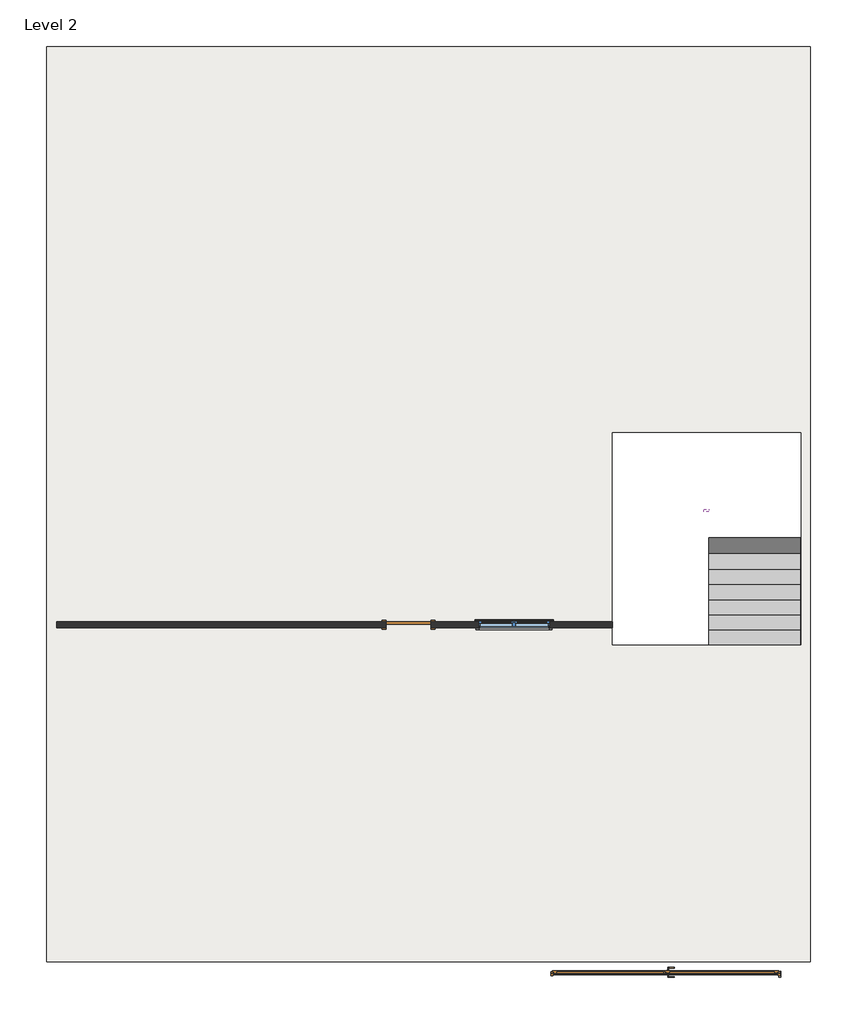
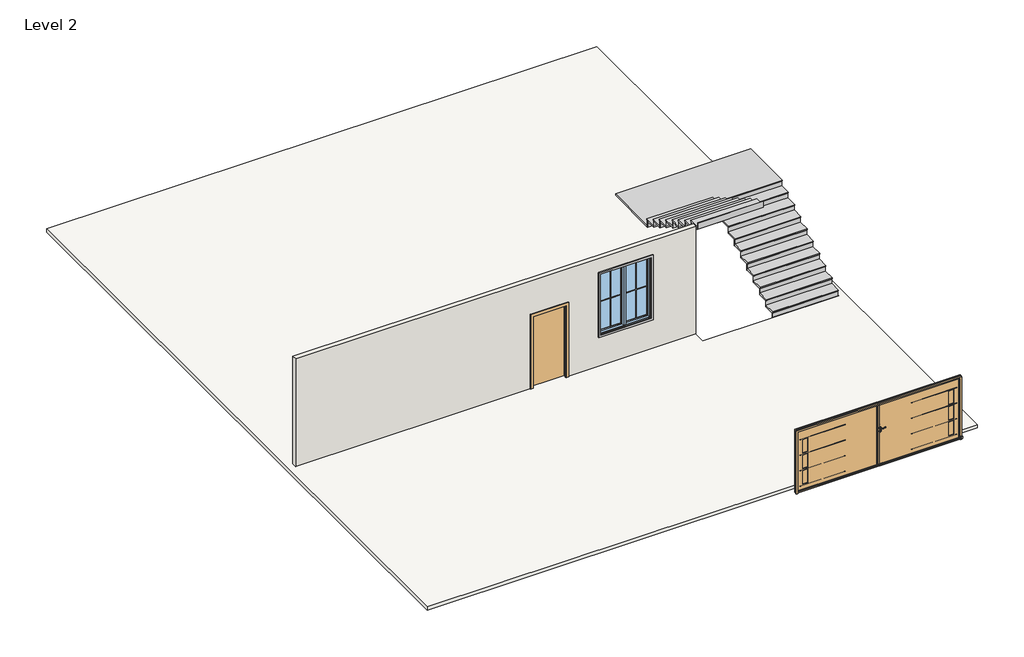
# One storey, incomplete: 4 proxies, 2 doors, 2 walls, 1 member, 1 slab, 1 stair flight, 1 window.
"""IFC4 building model written with IfcOpenShell, lengths in millimetres."""

from ifc_helpers import new_model, si_unit, frame, origin, place, context, project, spatial, polyline, outline, extrude, transform, mapped, element, save
from components import muntin_pattern_2x2_muntin_pattern_2x2_bff912c5, muntin_pattern_2x2_muntin_pattern_2x2_c2194282, trim_window_exterior_flat_with_sill_a4fd29d2, trim_window_interior_flat_picture_frame_640e2092, door_2a186d26, door_a3eb833a, stair_flight_26a2e14d, window_01a3843f

model = new_model("IFC4")

# Units and contexts
model_context = context("Model", 3, world=origin())
ifc_project = project(units=[si_unit("LENGTHUNIT", "METRE", prefix="MILLI")], contexts=[model_context])

# Site, building, storey
site = spatial("IfcSite", under=ifc_project)
building = spatial("IfcBuilding", under=site)
storey = spatial("IfcBuildingStorey", under=building, Name="Level 2", Elevation=762.0)

# Proxies
placement = place(None, origin())
muntin_pattern_2x2_muntin_pattern_2x2_shape = muntin_pattern_2x2_muntin_pattern_2x2_bff912c5(model_context)
element("IfcBuildingElementProxy", 1, Name="Muntin Pattern_2x2 : Muntin Pattern_2x2", ObjectType="Muntin Pattern_2x2 : Muntin Pattern_2x2", at=placement, inside=storey, context=model_context, shape_type="MappedRepresentation", body=[
    mapped(muntin_pattern_2x2_muntin_pattern_2x2_shape, transform((1639.5268946, -8189.1580955, 1746.25), x_axis=(1.0, 0.0, 0.0), y_axis=(0.0, 1.0, 0.0), z_axis=(0.0, 0.0, 1.0))),
])
muntin_pattern_2x2_muntin_pattern_2x2_2_shape = muntin_pattern_2x2_muntin_pattern_2x2_c2194282(model_context)
element("IfcBuildingElementProxy", 2, Name="Muntin Pattern_2x2 : Muntin Pattern_2x2", ObjectType="Muntin Pattern_2x2 : Muntin Pattern_2x2", at=placement, inside=storey, context=model_context, shape_type="MappedRepresentation", body=[
    mapped(muntin_pattern_2x2_muntin_pattern_2x2_2_shape, transform((2360.2518946, -8189.1580955, 1746.25), x_axis=(-1.0, 0.0, 0.0), y_axis=(0.0, -1.0, 0.0), z_axis=(0.0, 0.0, 1.0))),
])
trim_window_exterior_flat_with_sill_shape = trim_window_exterior_flat_with_sill_a4fd29d2(model_context)
element("IfcBuildingElementProxy", 3, Name="Trim-Window-Exterior-Flat : with Sill", ObjectType="Trim-Window-Exterior-Flat : with Sill", at=placement, inside=storey, context=model_context, shape_type="MappedRepresentation", body=[
    mapped(trim_window_exterior_flat_with_sill_shape, transform((1999.8893946, -8179.6330955, 3505.2), x_axis=(1.0, 0.0, 0.0), y_axis=(0.0, 0.0, -1.0), z_axis=(0.0, 1.0, 0.0))),
])
trim_window_interior_flat_picture_frame_shape = trim_window_interior_flat_picture_frame_640e2092(model_context)
element("IfcBuildingElementProxy", 4, Name="Trim-Window-Interior-Flat : Picture Frame", ObjectType="Trim-Window-Interior-Flat : Picture Frame", at=placement, inside=storey, context=model_context, shape_type="MappedRepresentation", body=[
    mapped(trim_window_interior_flat_picture_frame_shape, transform((1999.8893946, -8306.6330955, 3505.2), x_axis=(-1.0, 0.0, 0.0), y_axis=(0.0, 0.0, -1.0), z_axis=(0.0, -1.0, 0.0))),
])

# Doors
door_shape = door_2a186d26(model_context)
element("IfcDoor", 5, at=placement, inside=storey, context=model_context, shape_type="MappedRepresentation", body=[
    mapped(door_shape, transform((5061.1313124, -15304.3330955, 711.2), x_axis=(1.0, 0.0, 0.0), y_axis=(0.0, 1.0, 0.0), z_axis=(0.0, 0.0, 1.0))),
])
door_2_shape = door_a3eb833a(model_context)
element("IfcDoor", 6, ObjectType="Single-Flush : 36\" x 84\"", at=placement, inside=storey, context=model_context, shape_type="MappedRepresentation", body=[
    mapped(door_2_shape, transform((-133.7106054, -8243.1330955, 762.0), x_axis=(-1.0, 0.0, 0.0), y_axis=(0.0, -1.0, 0.0), z_axis=(0.0, 0.0, 1.0))),
])

# Member
element("IfcMember", 7, ObjectType="Stringer - 2\" Width", at=placement, inside=storey, context=model_context, shape_type="SweptSolid", body=[
    extrude(outline(polyline([(5940.6255016, -5904.9976656), (5940.6255016, -5955.7976656), (5839.0255016, -5955.7976656), (5839.0255016, -5904.9976656), (5940.6255016, -5904.9976656)])), frame((0.0, 0.0, 2311.4), z_axis=(0.0, 0.0, 1.0), x_axis=(1.0, 0.0, 0.0)), (0.0, 0.0, 1.0), 304.8),
])

# Slab
element("IfcSlab", 8, ObjectType="Generic - 4\"", at=placement, inside=storey, context=model_context, shape_type="SweptSolid", body=[
    extrude(outline(polyline([(-7454.7186876, -15050.3330955), (-7454.7186876, 3440.8669045), (7988.4813124, 3440.8669045), (7988.4813124, -15050.3330955), (-7454.7186876, -15050.3330955)]), holes=[polyline([(7797.9813124, -4367.7173694), (3981.0893946, -4367.7173694), (3981.0893946, -8648.1976656), (7797.9813124, -8648.1976656), (7797.9813124, -4367.7173694)])]), frame((0.0, 0.0, 660.4), z_axis=(0.0, 0.0, 1.0), x_axis=(1.0, 0.0, 0.0)), (0.0, 0.0, 1.0), 101.6),
])

# Stair flight
stair_flight_shape = stair_flight_26a2e14d(model_context)
element("IfcStairFlight", 9, ObjectType="2\" Tread 1\" Nosing 1/4\" Riser", at=placement, inside=storey, context=model_context, shape_type="MappedRepresentation", body=[
    mapped(stair_flight_shape, transform((0.0, 0.0, 0.0), x_axis=(1.0, 0.0, 0.0), y_axis=(0.0, 1.0, 0.0), z_axis=(0.0, 0.0, 1.0))),
])

# Walls
element("IfcWall", 10, ObjectType="Generic - 5\"", at=placement, inside=storey, context=model_context, shape_type="SweptSolid", body=[
    extrude(outline(polyline([(762.0, -7251.5186876), (762.0, -590.9106054), (2895.6, -590.9106054), (2895.6, 323.4893946), (762.0, 323.4893946), (762.0, 3981.0893946), (3962.4, 3981.0893946), (3962.4, -7251.5186876), (762.0, -7251.5186876)]), holes=[polyline([(3505.2, 1275.9893946), (3505.2, 2723.7893946), (1676.4, 2723.7893946), (1676.4, 1275.9893946), (3505.2, 1275.9893946)])]), frame((0.0, -8306.6330955, 0.0), z_axis=(0.0, 1.0, 0.0), x_axis=(0.0, 0.0, 1.0)), (0.0, 0.0, 1.0), 127.0),
])
element("IfcWall", 11, ObjectType="Generic - 5\"", at=placement, inside=storey, context=model_context, shape_type="SweptSolid", body=[
    extrude(outline(polyline([(7389.3205296, -15240.8330955), (7389.3205296, -15367.8330955), (7346.1313124, -15367.8330955), (7346.1313124, -15338.299607), (7380.1313124, -15338.299607), (7380.1313124, -15240.8330955), (7389.3205296, -15240.8330955)])), frame((0.0, 0.0, 762.0), z_axis=(0.0, 0.0, 1.0), x_axis=(1.0, 0.0, 0.0)), (0.0, 0.0, 1.0), 56.6987507),
])

# Window
window_shape = window_01a3843f(model_context)
element("IfcWindow", 12, ObjectType="Window-Casement-Double : 57\" x 72\"", at=placement, inside=storey, context=model_context, shape_type="MappedRepresentation", body=[
    mapped(window_shape, transform((1999.8893946, -8243.1330955, 762.0), x_axis=(-1.0, 0.0, 0.0), y_axis=(0.0, -1.0, 0.0), z_axis=(0.0, 0.0, 1.0))),
])

save(model, "model.ifc")

# Revit data of these elements
# Type "Muntin Pattern_2x2 : Muntin Pattern_2x2"
#   Width [instance default] = 4' - 0"
#   Thickness = 0' - 0 1/2"
#   Height [instance default] = 4' - 0"
#   Distance = 0' - 0 3/4"
#   Interior Material [instance default] = none
#   Exterior Material [instance default] = none
#   Default Elevation = 0
# Type "Trim-Window-Exterior-Flat : with Sill"
#   Trim Width = 0' - 2 1/4"
#   Trim Thickness_Picture Frame = 0' - 1 1/4"
#   Trim Thickness_with Sill = 0' - 0 3/4"
#   Sill Thickness = 0' - 1 1/4"
#   Opening Width [instance default] = 2' - 0"
#   Opening Height [instance default] = 3' - 0"
#   Default Elevation = 4' - 0"
#   Sill = yes
#   Picture Frame = no
#   Trim Material [instance default] = none
# Type "Trim-Window-Interior-Flat : Picture Frame"
#   Trim Thickness_Picture Frame = 0' - 1 1/4"
#   Trim Width = 0' - 2 1/4"
#   Trim Thickness_with Sill = 0' - 0 3/4"
#   Sill Thickness = 0' - 1 1/4"
#   Opening Width [instance default] = 2' - 0"
#   Opening Height [instance default] = 3' - 0"
#   Default Elevation = 4' - 0"
#   Sill = no
#   Picture Frame = yes
#   Trim Material [instance default] = none
# Type
#   Type Mark = "8"
#   Version Revit = "Revit 2017"
#   Uniformat II description = "Double door"
#   Uniformat CSI = "B2030"
#   URL = "https://www.fenetremeo.com/porte-entree"
#   Type de pose = "Tunnel"
#   Référence modèle = "MeO-PE-BALADE-2vtx"
#   Pose vitrage = "Vitrage collé"
#   Keynote = "MeO-PE-BALADE-2vtx"
#   Neuf / Réno = "Rénovation"
#   Model = "Porte double BALADE"
#   Matériaux = "Aluminium / bois"
#   IFC version = "IFC 2x3 Coordination 2.0"
#   IFC classification = "Door"
#   Fiches produits = "https://www.fenetremeo.com/porte-entree"
#   Famille de produit = "Porte"
#   Manufacturer = "MéO"
#   FILE_NAME = "2021-07-MeO-PE-BALADE-2vtx"
#   Design = "Modélisation non contractuelle"
#   Description = "Porte 2 vantaux égaux"
#   Contraintes largeur porte = "700 < Largeur < 1200"
#   Contraintes hauteur porte = "1953 < Hauteur < 2500"
#   Contraintes hauteur poignée porte = "900 <Hauteur poignée < 1300"
#   Analytic Construction = "<Aucun>"
#   Coefficient thermique Ud = "0.72 / 0.75 Ud"
#   BIMobject main category = "Exterior carpentry"
#   Avis technique = "https://www.fcba.fr/wp-content/uploads/2020/10/rc_nf297.pdf"
#   Surface = 27432' - 0"
#   Pose tunnel = 0' - 0.3937"
#   Longueur de traverse haute 33,43,53,63,73,83 = 0' - 1.29921"
#   Largeur zone 2 = 3' - 3.37008"
#   Largeur zone 1 = 3' - 3.37008"
#   Largeur du dormant 33,43,53,63,73,83 = 0' - 1.29921"
#   Rough Width = 15' - 2.59843"
#   Hauteur poignée = 3' - 7.30709"
#   Hauteur dormant = 6' - 1.33858"
#   Rough Height = 6' - 1.33858"
#   HT ouvrant = 5' - 11.25197"
#   Height = 6' - 0"
#   Width = 15' - 0"
#   Doublage 75,105,125,145,165,185,205 = 0' - 3.44356"
#   Message Hors abaques = yes
#   Hors abaques = yes
#   Vitrage = Verre
#   Couleur poignée = Acier inoxydable AISI 304
#   Choix du modèle = element 399147
#   Function = (empty or 0)
#   Wall Closure = (empty or 0)
# Type "Single-Flush : 36\" x 84\""
#   Type Mark = "1"
#   Construction Type Id = "MDOOR"
#   Assembly Code = "C1020"
#   Analytic Construction = "Metal"
#   Thickness = 0' - 2"
#   Heat Transfer Coefficient (U) = 0.651978 BTU/(h·ft²·°F)
#   Height = 7' - 0"
#   Trim Projection Ext = 0' - 1"
#   Trim Projection Int = 0' - 1"
#   Trim Width = 0' - 3"
#   Width = 3' - 0"
#   Define Thermal Properties by = 1
#   Define Thermal Properties by = 1
#   Door Material = Door - Panel
#   Frame Material = Door - Frame
#   Visual Light Transmittance = 0
#   Solar Heat Gain Coefficient = 0
#   Function = (empty or 0)
#   Wall Closure = (empty or 0)
# Type "Generic - 4\""
#   Assembly Code = "B1010"
#   Function = 0
#   Layers, outside or top first: 0' - 4" no material (function 1)
# Type "Generic - 5\""
#   Assembly Code = "B2010"
#   Layers, outside or top first: 0' - 5" no material (function 1)
# Type "Window-Casement-Double : 57\" x 72\""
#   Type Mark = "17"
#   Fire Rating = "0.5h"
#   Assembly Code = "B2020100"
#   Analytic Construction = "Double glazing - domestic"
#   Frame Extension [instance default] = 0' - 0 1/4"
#   Window Inset [instance default] = 0' - 0"
#   Wall Thickness [instance default] = 0' - 6"
#   Interior Wall Closure [instance default] = 0' - 2 1/4"
#   Half Width = 2' - 4 1/2"
#   Visual Light Transmittance = 0.81
#   Thermal Resistance (R) = 1.8146 (h·ft²·°F)/BTU
#   Solar Heat Gain Coefficient = 0.76
#   Rough Width = 4' - 9 1/2"
#   Rough Height = 6' - 0 1/2"
#   Height = 6' - 0"
#   Heat Transfer Coefficient (U) = 0.5511 BTU/(h·ft²·°F)
#   Exterior Wall Closure [instance default] = 0' - 1 1/4"
#   Extension Jamb [instance default] = 0' - 2 1/4"
#   Default Sill Height = 3' - 0"
#   Width = 4' - 9"
#   Define Thermal Properties by = 0
#   Muntin Visibility = yes
#   Interior Trim Visibility [instance default] = yes
#   Exterior Trim Visibility [instance default] = yes
#   Extension Jamb Visibility [instance default] = yes
#   Interior Trim Material = Wood - Stained
#   Muntin Pattern = Muntin Pattern_2x2 : Muntin Pattern_2x2
#   Interior Trim = Trim-Window-Interior-Flat : Picture Frame
#   Interior Frame Material = Wood - Stained
#   Glass Panel Material = Glass
#   Exterior Trim Material = Clad - White
#   Exterior Trim = Trim-Window-Exterior-Flat : with Sill
#   Exterior Frame Material = Clad - White
#   Wall Closure = (empty or 0)
# Elements 1, 2 (IfcBuildingElementProxy, "Muntin Pattern_2x2 : Muntin Pattern_2x2")
#   Width = 1' - 11 1/8"
#   Height = 5' - 6 1/2"
#   Interior Material = Wood - Stained
#   Exterior Material = Clad - White
#   Phase Created = New Construction
#   Materials on its faces: "Clad - White", "Wood - Stained"
# Element 3 (IfcBuildingElementProxy, "Trim-Window-Exterior-Flat : with Sill")
#   Opening Width = 4' - 9"
#   Opening Height = 6' - 0"
#   Trim Material = Clad - White
#   Phase Created = New Construction
#   Materials on its faces: "Clad - White"
# Element 4 (IfcBuildingElementProxy, "Trim-Window-Interior-Flat : Picture Frame")
#   Opening Width = 4' - 9"
#   Opening Height = 6' - 0"
#   Trim Material = Wood - Stained
#   Phase Created = New Construction
#   Materials on its faces: "Wood - Stained"
# Element 5 (IfcDoor)
#   Phase Created = New Construction
#   Materials on its faces: "Acier inoxydable AISI 304", "Verre", "Aluminium"
# Element 6 (IfcDoor, "Single-Flush : 36\" x 84\"")
#   Phase Created = New Construction
#   Materials on its faces: "Door - Frame", "Door - Panel"
# Element 7 (IfcMember, "Stringer - 2\" Width")
#   Phase Created = New Construction
# Element 8 (IfcSlab, "Generic - 4\"")
#   built-in parameter 1001955 = -1.5708 (stored number, unit not read)
#   Height Offset From Level = 0' - 0"
#   Phase Created = New Construction
#   Materials on its faces: "Default Floor", "floor"
# Element 9 (IfcStairFlight, "2\" Tread 1\" Nosing 1/4\" Riser")
#   Phase Created = New Construction
# Element 10 (IfcWall, "Generic - 5\"")
#   Top Offset = 0' - 0"
#   Base Offset = 0' - 0"
#   wall height = 10' - 6"
#   Phase Created = New Construction
#   Base Constraint = Level 2
#   Top Constraint = Level 3
#   Materials on its faces: "Default Wall"
# Element 11 (IfcWall, "Generic - 5\"")
#   Top Offset = 0' - 2.23223"
#   Base Offset = 0' - 0"
#   wall height = 0' - 2.23223"
#   Phase Created = New Construction
#   Base Constraint = Level 2
#   Top Constraint = Level 2
#   Materials on its faces: "Default Wall"
# Element 12 (IfcWindow, "Window-Casement-Double : 57\" x 72\"")
#   Mark = "1"
#   Window Inset = 0' - 0"
#   Interior Wall Closure = 0' - 2 1/4"
#   Frame Extension = 0' - 0 1/4"
#   Exterior Wall Closure = 0' - 1 1/4"
#   Interior Trim Visibility = yes
#   Exterior Trim Visibility = yes
#   Phase Created = New Construction
#   Materials on its faces: "Wood - Stained", "Glass", "Clad - White"
# Materials
#   "Verre": class "Verre", colour RGB 92 99 177, transparency 0.7, Description = "Verre sodocalcique", Cost = 0
#   "Acier inoxydable AISI 304": colour RGB 120 120 120, transparency 0, Description = "Stainless Steel 18/8", Cost = 0
#   "Door - Panel": class "Wood", colour RGB 210 159 95, transparency 0, Cost = 0
#   "Door - Frame": colour RGB 118 70 51, transparency 0, Cost = 0
#   "Wood - Stained": class "Wood", colour RGB 224 178 126, transparency 0, Cost = 0
#   "Glass": class "Glass", colour RGB 0 128 192, transparency 0.75, Description = "Soda Lime Glass", Cost = 0
#   "Clad - White": class "Wood", colour RGB 242 242 238, transparency 0, Cost = 0
#   "Aluminium": colour RGB 247 247 247, transparency 0, Description = "Aluminium 6061", Cost = 0
#   "Default Floor": colour RGB 128 128 128, transparency 0, Cost = 0
#   "floor": class "Generic", colour RGB 255 207 159, transparency 0, Cost = 0
#   "Default Wall": colour RGB 128 128 128, transparency 0, Cost = 0
